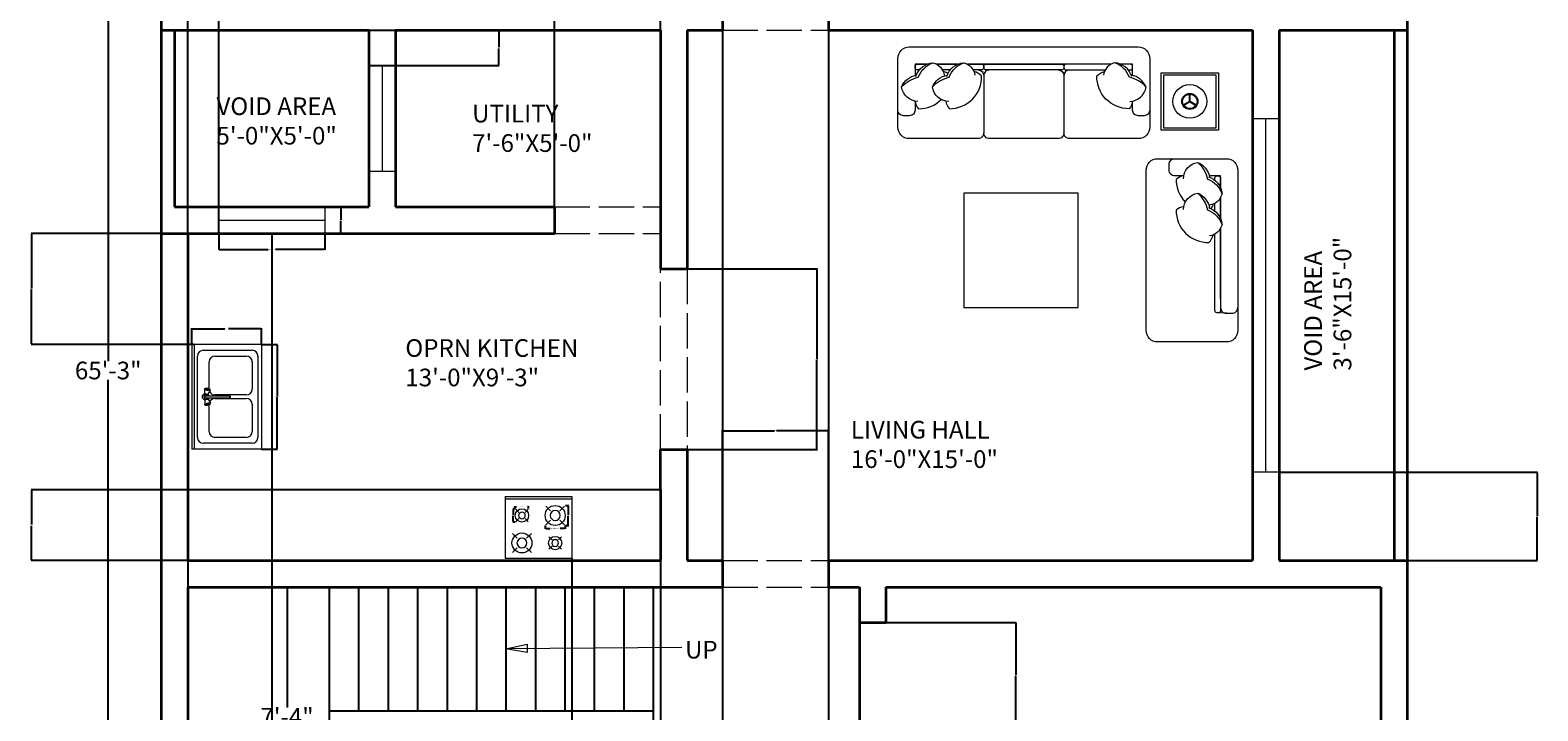
# Model space of a CAD drawing. Units: inches. Extents: x -10 to 502, y -868 to 56.
# Tile 9 of 14: x -10 to 502, y -495 to -264. Entities that reach past the tile are written whole.
import ezdxf

# ---------------------------------------------------------------- set-up
doc = ezdxf.new("R2010")
doc.units = ezdxf.units.IN
doc.header["$MEASUREMENT"] = 0
doc.linetypes.add('ACAD_ISO02W100', pattern=[15, 12, -3])
for name, color, linetype, lineweight in [('A-ANNO-DIMS', 2, 'Continuous', 18), ('A-ANNO-SYMB', 7, 'Continuous', 18), ('A-ANNO-TEXT', 7, 'Continuous', 18), ('A-AREA-IDEN', 7, 'Continuous', 18), ('A-EQPM', 8, 'Continuous', 18), ('A-FLOR-CASE', 8, 'Continuous', 18), ('A-FLOR-FIXT', 8, 'Continuous', 18), ('A-FLOR-STRS', 7, 'Continuous', 25), ('A-FURN', 8, 'Continuous', 13), ('A-GLAZ', 162, 'Continuous', 18), ('A-WALL', 7, 'Continuous', 35), ('A-WALL-OVHD', 7, 'ACAD_ISO02W100', 18)]:
    doc.layers.add(name, color=color, linetype=linetype, lineweight=lineweight)
doc.styles.get("Standard").update_dxf_attribs({"font": 'arial.ttf'})
doc.dimstyles.get("Standard").update_dxf_attribs({"dimtxt": 0.18, "dimasz": 0.18, "dimexe": 0.18, "dimexo": 0.0625, "dimgap": 0.09, "dimtad": 0, "dimtih": 1, "dimtoh": 1, "dimdec": 0, "dimzin": 0, "dimdsep": 46, "dimlunit": 3, "dimtxsty": 'Standard', "dimcen": 0.09, "dimadec": 0, "dimazin": 0, "dimtfac": 1, "dimtdec": 0, "dimtofl": 0, "dimtmove": 0, "dimatfit": 3, "dimfxl": 1, "dimtolj": 1, "dimtzin": 0, "dimarcsym": 0})

# ---------------------------------------------------------------- blocks, each defined once
blk = doc.blocks.new('*D2')
at = {"layer": 'A-ANNO-DIMS', "color": 0, "lineweight": -2, "transparency": 16777216}
for p, q in [((34.89, 12.15), (16.75, 12.15)), ((16.93, 11.97), (16.93, -376.2)), ((16.93, -770.67), (16.93, -382.51)), ((34.89, -770.85), (16.75, -770.85))]:
    blk.add_line(p, q, dxfattribs=at)
at = {"layer": 'A-ANNO-DIMS', "color": 0, "transparency": 16777216}
for points in [[(16.9, 11.97), (16.96, 11.97), (16.93, 12.15)], [(16.9, -770.67), (16.96, -770.67), (16.93, -770.85)]]:
    blk.add_solid(points, dxfattribs=at)
at = {"layer": 'Defpoints', "color": 0, "transparency": 16777216}
for p in [(34.95, 12.15), (16.93, -770.85), (34.95, -770.85)]:
    blk.add_point(p, dxfattribs=at)
at = {"layer": 'A-ANNO-DIMS', "color": 0, "transparency": 16777216, "insert": (16.93, -379.35), "char_height": 6, "attachment_point": 5}
blk.add_mtext('\\A1;65\'-3"', dxfattribs=at)
blk = doc.blocks.new('М07 600х900')
for p, q in [((0, 600), (-900, 600)), ((-900, 0), (-900, 600)), ((-900, 0), (-900, 600)), ((0, 580), (-900, 580)), ((-800, 550), (-100, 550)), ((0, 0), (0, 600)), ((0, 0), (0, 600)), ((-850, 80), (-850, 500)), ((-800, 130), (-800, 400)), ((-750, 450), (-519, 450)), ((-525, 477), (-524, 480)), ((-525, 472), (-525, 477)), ((-524, 466), (-525, 472)), ((-521, 486), (-524, 480)), ((-524, 480), (-522, 481)), ((-523, 460), (-524, 466)), ((-521, 455), (-523, 460)), ((-522, 481), (-520, 481)), ((-521, 486), (-519, 487)), ((-519, 449), (-521, 455)), ((-520, 481), (-518, 479)), ((-480, 488), (-519, 487)), ((-519, 487), (-516, 487)), ((-516, 445), (-519, 449)), ((-518, 479), (-515, 475)), ((-516, 487), (-513, 484)), ((-514, 443), (-516, 445)), ((-515, 475), (-513, 470)), ((-509, 440), (-514, 443)), ((-512, 443), (-514, 443)), ((-513, 484), (-510, 479)), ((-513, 470), (-511, 464)), ((-510, 444), (-512, 443)), ((-511, 464), (-510, 458)), ((-510, 479), (-507, 473)), ((-510, 458), (-509, 452)), ((-509, 447), (-510, 444)), ((-509, 452), (-509, 447)), ((-506, 439), (-509, 440)), ((-507, 473), (-505, 465)), ((-472, 459), (-506, 439)), ((-504, 441), (-506, 439)), ((-505, 465), (-503, 458)), ((-503, 445), (-504, 441)), ((-503, 458), (-503, 451)), ((-503, 451), (-503, 445)), ((-480, 488), (-478, 487)), ((-478, 487), (-476, 486)), ((-477, 489), (-473, 496)), ((-477, 486), (-477, 489)), ((-461, 489), (-476, 485)), ((-476, 486), (-474, 483)), ((-474, 483), (-473, 479)), ((-473, 496), (-466, 503)), ((-473, 479), (-471, 474)), ((-471, 460), (-472, 459)), ((-471, 474), (-470, 470)), ((-470, 462), (-471, 460)), ((-470, 470), (-470, 466)), ((-470, 466), (-470, 462)), ((-458, 465), (-470, 462)), ((-466, 457), (-470, 461)), ((-466, 503), (-459, 507)), ((-459, 453), (-466, 457)), ((-465, 480), (-462, 489)), ((-462, 471), (-465, 480)), ((-465, 400), (-465, 130)), ((-462, 489), (-455, 494)), ((-458, 469), (-462, 471)), ((-459, 507), (-450, 508)), ((-458, 453), (-459, 453)), ((-458, 480), (-457, 485)), ((-458, 480), (-458, 280)), ((-457, 485), (-453, 488)), ((-455, 494), (-445, 494)), ((-453, 488), (-447, 488)), ((-450, 508), (-441, 507)), ((-447, 488), (-443, 485)), ((-445, 494), (-438, 489)), ((-443, 485), (-442, 480)), ((-442, 480), (-442, 280)), ((-438, 471), (-442, 469)), ((-442, 465), (-430, 462)), ((-441, 453), (-442, 453)), ((-441, 507), (-434, 503)), ((-434, 457), (-441, 453)), ((-439, 489), (-424, 485)), ((-438, 489), (-435, 480)), ((-435, 480), (-438, 471)), ((-435, 130), (-435, 400)), ((-434, 503), (-427, 496)), ((-430, 461), (-434, 457)), ((-430, 470), (-429, 474)), ((-430, 466), (-430, 470)), ((-430, 462), (-430, 466)), ((-429, 460), (-430, 462)), ((-429, 474), (-427, 479)), ((-428, 459), (-429, 460)), ((-428, 459), (-394, 439)), ((-427, 496), (-423, 489)), ((-427, 479), (-426, 483)), ((-426, 483), (-424, 486)), ((-424, 486), (-422, 487)), ((-423, 489), (-423, 486)), ((-422, 487), (-420, 488)), ((-420, 488), (-381, 487)), ((-397, 458), (-395, 465)), ((-397, 451), (-397, 458)), ((-397, 445), (-397, 451)), ((-396, 441), (-397, 445)), ((-394, 439), (-396, 441)), ((-395, 465), (-393, 473)), ((-391, 440), (-394, 439)), ((-393, 473), (-390, 479)), ((-391, 452), (-390, 458)), ((-391, 447), (-391, 452)), ((-390, 444), (-391, 447)), ((-391, 440), (-386, 443)), ((-390, 479), (-387, 484)), ((-390, 458), (-389, 464)), ((-388, 443), (-390, 444)), ((-389, 464), (-387, 470)), ((-386, 443), (-388, 443)), ((-387, 484), (-384, 487)), ((-387, 470), (-385, 475)), ((-384, 445), (-386, 443)), ((-385, 475), (-382, 479)), ((-384, 487), (-381, 487)), ((-381, 449), (-384, 445)), ((-382, 479), (-380, 481)), ((-381, 487), (-379, 486)), ((-379, 455), (-381, 449)), ((-381, 450), (-150, 450)), ((-380, 481), (-378, 481)), ((-379, 486), (-376, 480)), ((-377, 460), (-379, 455)), ((-378, 481), (-376, 480)), ((-376, 466), (-377, 460)), ((-376, 480), (-375, 477)), ((-375, 472), (-376, 466)), ((-375, 477), (-375, 472)), ((-100, 400), (-100, 130)), ((-50, 500), (-50, 80)), ((-458, 286), (-460, 280)), ((-460, 280), (-458, 274)), ((-458, 280), (-457, 275)), ((-458, 274), (-457, 270)), ((-458, 274), (-453, 271)), ((-457, 275), (-453, 272)), ((-457, 270), (-453, 267)), ((-453, 272), (-447, 272)), ((-453, 271), (-447, 271)), ((-453, 267), (-447, 267)), ((-447, 272), (-443, 275)), ((-447, 271), (-442, 274)), ((-447, 267), (-443, 270)), ((-443, 275), (-442, 280)), ((-442, 274), (-443, 270)), ((-440, 280), (-442, 286)), ((-442, 274), (-440, 280)), ((0, 0), (-900, 0)), ((-100, 30), (-800, 30)), ((-515, 80), (-750, 80)), ((-150, 80), (-385, 80))]:
    blk.add_line(p, q)
for centre, start, end in [((-800, 500), 90, 180), ((-100, 500), 0, 90), ((-750, 400), 90, 180), ((-515, 400), 0, 65.8874), ((-385, 400), 114.1126, 180), ((-150, 400), 0, 90), ((-750, 130), 180, 270), ((-515, 130), 270, 0), ((-385, 130), 180, 270), ((-150, 130), 270, 0), ((-800, 80), 180, 270), ((-100, 80), 270, 0)]:
    blk.add_arc(centre, 50, start, end)
for p in [(-515, 80), (-150, 80), (-100, 30)]:
    blk.add_point(p)
blk = doc.blocks.new('*D6')
at = {"layer": 'A-ANNO-DIMS', "color": 0, "lineweight": -2, "transparency": 16777216}
for p, q in [((76.89, -452.85), (77.81, -452.85)), ((77.63, -453.03), (77.63, -493.76)), ((77.63, -540.67), (77.63, -499.94)), ((76.89, -540.85), (77.81, -540.85))]:
    blk.add_line(p, q, dxfattribs=at)
at = {"layer": 'A-ANNO-DIMS', "color": 0, "transparency": 16777216}
for points in [[(77.6, -453.03), (77.66, -453.03), (77.63, -452.85)], [(77.6, -540.67), (77.66, -540.67), (77.63, -540.85)]]:
    blk.add_solid(points, dxfattribs=at)
at = {"layer": 'Defpoints', "color": 0, "transparency": 16777216}
for p in [(76.83, -452.85), (76.83, -540.85), (77.63, -540.85)]:
    blk.add_point(p, dxfattribs=at)
at = {"layer": 'A-ANNO-DIMS', "color": 0, "transparency": 16777216, "insert": (77.63, -496.85), "char_height": 6, "attachment_point": 5}
blk.add_mtext('\\A1;7\'-4"', dxfattribs=at)
blk = doc.blocks.new('WIN-36IN')
for p, q in [((0, 9), (36, 9)), ((0, 0), (0, 9)), ((36, 9), (36, 0)), ((0, 4.5), (36, 4.5)), ((36, 0), (0, 0))]:
    blk.add_line(p, q)
blk = doc.blocks.new('WIN-120IN')
for p, q in [((0, 9), (120, 9)), ((0, 0), (0, 9)), ((120, 9), (120, 0)), ((0, 4.5), (120, 4.5)), ((120, 0), (0, 0))]:
    blk.add_line(p, q)
blk = doc.blocks.new('COOKTOP-BURNER-SMALL')
for p, q in [((1.19, 3.32), (0.13, 4.39)), ((1.19, 1.19), (0.13, 0.13)), ((3.32, 3.32), (4.39, 4.39)), ((3.32, 1.19), (4.39, 0.13))]:
    blk.add_line(p, q)
blk.add_circle((2.26, 2.26), 2.26)
for start, end in [(0, 180), (180, 0)]:
    blk.add_arc((2.26, 2.26), 1.13, start, end)
blk = doc.blocks.new('COOKTOP-BURNER-LARGE')
for p, q in [((1.79, 4.98), (0.19, 6.58)), ((4.98, 4.98), (6.58, 6.58)), ((1.79, 1.79), (0.19, 0.19)), ((4.98, 1.79), (6.58, 0.19))]:
    blk.add_line(p, q)
blk.add_circle((3.39, 3.39), 3.39)
for start, end in [(0, 180), (180, 0)]:
    blk.add_arc((3.39, 3.39), 1.69, start, end)
blk = doc.blocks.new('*D17')
at = {"layer": 'A-ANNO-DIMS', "color": 0, "lineweight": -2, "transparency": 16777216}
for p, q in [((54.45, -332.92), (54.45, -338.43)), ((90.45, -332.92), (90.45, -338.43)), ((54.63, -338.25), (71.22, -338.25)), ((90.27, -338.25), (73.68, -338.25))]:
    blk.add_line(p, q, dxfattribs=at)
at = {"layer": 'A-ANNO-DIMS', "color": 0, "transparency": 16777216}
for points in [[(54.63, -338.22), (54.63, -338.28), (54.45, -338.25)], [(90.27, -338.22), (90.27, -338.28), (90.45, -338.25)]]:
    blk.add_solid(points, dxfattribs=at)
at = {"layer": 'Defpoints', "color": 0, "transparency": 16777216}
for p in [(54.45, -332.85), (90.45, -332.85), (90.45, -338.25)]:
    blk.add_point(p, dxfattribs=at)
at = {"layer": 'A-ANNO-DIMS', "color": 0, "transparency": 16777216, "insert": (72.45, -338.25), "char_height": 0.18, "attachment_point": 5}
blk.add_mtext('\\A1;WINDOW 3\'-0" TYP.', dxfattribs=at)
blk = doc.blocks.new('*D18')
at = {"layer": 'A-ANNO-DIMS', "color": 0, "lineweight": -2, "transparency": 16777216}
for p, q in [((90.51, -323.85), (96.03, -323.85)), ((95.85, -324.03), (95.85, -328.17)), ((95.85, -332.67), (95.85, -328.53)), ((90.51, -332.85), (96.03, -332.85))]:
    blk.add_line(p, q, dxfattribs=at)
at = {"layer": 'A-ANNO-DIMS', "color": 0, "transparency": 16777216}
for points in [[(95.82, -324.03), (95.88, -324.03), (95.85, -323.85)], [(95.82, -332.67), (95.88, -332.67), (95.85, -332.85)]]:
    blk.add_solid(points, dxfattribs=at)
at = {"layer": 'Defpoints', "color": 0, "transparency": 16777216}
for p in [(90.45, -323.85), (95.85, -323.85), (90.45, -332.85)]:
    blk.add_point(p, dxfattribs=at)
at = {"layer": 'A-ANNO-DIMS', "color": 0, "transparency": 16777216, "insert": (95.85, -328.35), "char_height": 0.18, "attachment_point": 5}
blk.add_mtext('\\A1;0\'-9" TYP.', dxfattribs=at)
blk = doc.blocks.new('*D33')
at = {"layer": 'A-ANNO-DIMS', "color": 0, "lineweight": -2, "transparency": 16777216}
for p, q in [((69.01, -370.51), (74.45, -370.51)), ((74.27, -370.69), (74.27, -388.07)), ((74.27, -405.82), (74.27, -388.44)), ((69.01, -406), (74.45, -406))]:
    blk.add_line(p, q, dxfattribs=at)
at = {"layer": 'A-ANNO-DIMS', "color": 0, "transparency": 16777216}
for points in [[(74.24, -370.69), (74.3, -370.69), (74.27, -370.51)], [(74.24, -405.82), (74.3, -405.82), (74.27, -406)]]:
    blk.add_solid(points, dxfattribs=at)
at = {"layer": 'Defpoints', "color": 0, "transparency": 16777216}
for p in [(68.94, -370.51), (74.27, -370.51), (68.94, -406)]:
    blk.add_point(p, dxfattribs=at)
at = {"layer": 'A-ANNO-DIMS', "color": 0, "transparency": 16777216, "insert": (74.27, -388.26), "char_height": 0.18, "attachment_point": 5}
blk.add_mtext('\\A1;SINK 2\'-11 1/2"', dxfattribs=at)
blk = doc.blocks.new('*D34')
at = {"layer": 'A-ANNO-DIMS', "color": 0, "lineweight": -2, "transparency": 16777216}
for p, q in [((45.28, -370.45), (45.28, -365)), ((45.46, -365.18), (56.51, -365.18)), ((68.76, -365.18), (57.71, -365.18)), ((68.94, -370.45), (68.94, -365))]:
    blk.add_line(p, q, dxfattribs=at)
at = {"layer": 'A-ANNO-DIMS', "color": 0, "transparency": 16777216}
for points in [[(45.46, -365.15), (45.46, -365.21), (45.28, -365.18)], [(68.76, -365.15), (68.76, -365.21), (68.94, -365.18)]]:
    blk.add_solid(points, dxfattribs=at)
at = {"layer": 'Defpoints', "color": 0, "transparency": 16777216}
for p in [(45.28, -365.18), (45.28, -370.51), (68.94, -370.51)]:
    blk.add_point(p, dxfattribs=at)
at = {"layer": 'A-ANNO-DIMS', "color": 0, "transparency": 16777216, "insert": (57.11, -365.18), "char_height": 0.18, "attachment_point": 5}
blk.add_mtext('\\A1;1\'-11 1/2"', dxfattribs=at)
blk = doc.blocks.new('*D37')
at = {"layer": 'A-ANNO-DIMS', "color": 0, "lineweight": -2, "transparency": 16777216}
for p, q in [((155.13, -426.23), (155.13, -425.44)), ((155.31, -425.62), (155.53, -425.62)), ((159.46, -425.62), (159.25, -425.62)), ((159.64, -426.23), (159.64, -425.44))]:
    blk.add_line(p, q, dxfattribs=at)
at = {"layer": 'A-ANNO-DIMS', "color": 0, "transparency": 16777216}
for points in [[(155.31, -425.59), (155.31, -425.65), (155.13, -425.62)], [(159.46, -425.59), (159.46, -425.65), (159.64, -425.62)]]:
    blk.add_solid(points, dxfattribs=at)
at = {"layer": 'Defpoints', "color": 0, "transparency": 16777216}
for p in [(155.13, -426.29), (159.64, -425.62), (159.64, -426.29)]:
    blk.add_point(p, dxfattribs=at)
at = {"layer": 'A-ANNO-DIMS', "color": 0, "transparency": 16777216, "insert": (157.39, -425.62), "char_height": 0.18, "attachment_point": 5}
blk.add_mtext('\\A1;SMALL BURNER 0\'-4 1/2" TYP.', dxfattribs=at)
blk = doc.blocks.new('*D38')
at = {"layer": 'A-ANNO-DIMS', "color": 0, "lineweight": -2, "transparency": 16777216}
for p, q in [((155.07, -426.29), (154.27, -426.29)), ((154.45, -426.47), (154.45, -428.37)), ((154.45, -430.63), (154.45, -428.73)), ((155.07, -430.81), (154.27, -430.81))]:
    blk.add_line(p, q, dxfattribs=at)
at = {"layer": 'A-ANNO-DIMS', "color": 0, "transparency": 16777216}
for points in [[(154.42, -426.47), (154.48, -426.47), (154.45, -426.29)], [(154.42, -430.63), (154.48, -430.63), (154.45, -430.81)]]:
    blk.add_solid(points, dxfattribs=at)
at = {"layer": 'Defpoints', "color": 0, "transparency": 16777216}
for p in [(154.45, -426.29), (155.13, -426.29), (155.13, -430.81)]:
    blk.add_point(p, dxfattribs=at)
at = {"layer": 'A-ANNO-DIMS', "color": 0, "transparency": 16777216, "insert": (154.45, -428.55), "char_height": 0.18, "attachment_point": 5}
blk.add_mtext('\\A1;0\'-4 1/2" TYP.', dxfattribs=at)
blk = doc.blocks.new('*D39')
at = {"layer": 'A-ANNO-DIMS', "color": 0, "lineweight": -2, "transparency": 16777216}
for p, q in [((165.29, -432), (165.29, -433.13)), ((165.47, -432.95), (167.01, -432.95)), ((171.88, -432.95), (170.34, -432.95)), ((172.06, -432), (172.06, -433.13))]:
    blk.add_line(p, q, dxfattribs=at)
at = {"layer": 'A-ANNO-DIMS', "color": 0, "transparency": 16777216}
for points in [[(165.47, -432.92), (165.47, -432.98), (165.29, -432.95)], [(171.88, -432.92), (171.88, -432.98), (172.06, -432.95)]]:
    blk.add_solid(points, dxfattribs=at)
at = {"layer": 'Defpoints', "color": 0, "transparency": 16777216}
for p in [(165.29, -431.94), (165.29, -432.95), (172.06, -431.94)]:
    blk.add_point(p, dxfattribs=at)
at = {"layer": 'A-ANNO-DIMS', "color": 0, "transparency": 16777216, "insert": (168.68, -432.95), "char_height": 0.18, "attachment_point": 5}
blk.add_mtext('\\A1;LARGE BURNER 0\'-7" TYP.', dxfattribs=at)
blk = doc.blocks.new('*D40')
at = {"layer": 'A-ANNO-DIMS', "color": 0, "lineweight": -2, "transparency": 16777216}
for p, q in [((172.12, -425.16), (173.26, -425.16)), ((173.08, -425.34), (173.08, -428.37)), ((173.08, -431.76), (173.08, -428.73)), ((172.12, -431.94), (173.26, -431.94))]:
    blk.add_line(p, q, dxfattribs=at)
at = {"layer": 'A-ANNO-DIMS', "color": 0, "transparency": 16777216}
for points in [[(173.05, -425.34), (173.11, -425.34), (173.08, -425.16)], [(173.05, -431.76), (173.11, -431.76), (173.08, -431.94)]]:
    blk.add_solid(points, dxfattribs=at)
at = {"layer": 'Defpoints', "color": 0, "transparency": 16777216}
for p in [(172.06, -425.16), (172.06, -431.94), (173.08, -431.94)]:
    blk.add_point(p, dxfattribs=at)
at = {"layer": 'A-ANNO-DIMS', "color": 0, "transparency": 16777216, "insert": (173.08, -428.55), "char_height": 0.18, "attachment_point": 5}
blk.add_mtext('\\A1;0\'-7" TYP.', dxfattribs=at)
blk = doc.blocks.new('*D48')
at = {"layer": 'A-ANNO-DIMS', "color": 0, "lineweight": -2, "transparency": 16777216}
for p, q in [((43.95, -332.92), (43.95, -846.58)), ((72.45, -332.92), (72.45, -846.58)), ((44.13, -846.4), (57.66, -846.4)), ((72.27, -846.4), (58.74, -846.4))]:
    blk.add_line(p, q, dxfattribs=at)
at = {"layer": 'A-ANNO-DIMS', "color": 0, "transparency": 16777216}
for points in [[(44.13, -846.37), (44.13, -846.43), (43.95, -846.4)], [(72.27, -846.37), (72.27, -846.43), (72.45, -846.4)]]:
    blk.add_solid(points, dxfattribs=at)
at = {"layer": 'Defpoints', "color": 0, "transparency": 16777216}
for p in [(43.95, -332.85), (72.45, -332.85), (72.45, -846.4)]:
    blk.add_point(p, dxfattribs=at)
at = {"layer": 'A-ANNO-DIMS', "color": 0, "transparency": 16777216, "insert": (58.2, -846.4), "char_height": 0.18, "attachment_point": 5}
blk.add_mtext('\\A1;2\'-4 1/2"', dxfattribs=at)
blk = doc.blocks.new('*D49')
at = {"layer": 'A-ANNO-DIMS', "color": 0, "lineweight": -2, "transparency": 16777216}
for p, q in [((204.39, -419.85), (-9.28, -419.85)), ((-9.1, -420.03), (-9.1, -431.67)), ((-9.1, -443.67), (-9.1, -432.03)), ((204.39, -443.85), (-9.28, -443.85))]:
    blk.add_line(p, q, dxfattribs=at)
at = {"layer": 'A-ANNO-DIMS', "color": 0, "transparency": 16777216}
for points in [[(-9.13, -420.03), (-9.07, -420.03), (-9.1, -419.85)], [(-9.13, -443.67), (-9.07, -443.67), (-9.1, -443.85)]]:
    blk.add_solid(points, dxfattribs=at)
at = {"layer": 'Defpoints', "color": 0, "transparency": 16777216}
for p in [(204.45, -419.85), (-9.1, -443.85), (204.45, -443.85)]:
    blk.add_point(p, dxfattribs=at)
at = {"layer": 'A-ANNO-DIMS', "color": 0, "transparency": 16777216, "insert": (-9.1, -431.85), "char_height": 0.18, "attachment_point": 5}
blk.add_mtext('\\A1;2\'-0"', dxfattribs=at)
blk = doc.blocks.new('*D52')
at = {"layer": 'A-ANNO-DIMS', "color": 0, "lineweight": -2, "transparency": 16777216}
for p, q in [((414.51, -413.85), (502.18, -413.85)), ((502, -414.03), (502, -428.67)), ((502, -443.67), (502, -429.03)), ((414.51, -443.85), (502.18, -443.85))]:
    blk.add_line(p, q, dxfattribs=at)
at = {"layer": 'A-ANNO-DIMS', "color": 0, "transparency": 16777216}
for points in [[(501.97, -414.03), (502.03, -414.03), (502, -413.85)], [(501.97, -443.67), (502.03, -443.67), (502, -443.85)]]:
    blk.add_solid(points, dxfattribs=at)
at = {"layer": 'Defpoints', "color": 0, "transparency": 16777216}
for p in [(414.45, -413.85), (414.45, -443.85), (502, -443.85)]:
    blk.add_point(p, dxfattribs=at)
at = {"layer": 'A-ANNO-DIMS', "color": 0, "transparency": 16777216, "insert": (502, -428.85), "char_height": 0.18, "attachment_point": 5}
blk.add_mtext('\\A1;2\'-6"', dxfattribs=at)
blk = doc.blocks.new('*D53')
at = {"layer": 'A-ANNO-DIMS', "color": 0, "lineweight": -2, "transparency": 16777216}
for p, q in [((174.32, -443.06), (174.32, -846.58)), ((204.45, -443.92), (204.45, -846.58)), ((174.5, -846.4), (189.05, -846.4)), ((204.27, -846.4), (189.72, -846.4))]:
    blk.add_line(p, q, dxfattribs=at)
at = {"layer": 'A-ANNO-DIMS', "color": 0, "transparency": 16777216}
for points in [[(174.5, -846.37), (174.5, -846.43), (174.32, -846.4)], [(204.27, -846.37), (204.27, -846.43), (204.45, -846.4)]]:
    blk.add_solid(points, dxfattribs=at)
at = {"layer": 'Defpoints', "color": 0, "transparency": 16777216}
for p in [(174.32, -443), (204.45, -443.85), (204.45, -846.4)]:
    blk.add_point(p, dxfattribs=at)
at = {"layer": 'A-ANNO-DIMS', "color": 0, "transparency": 16777216, "insert": (189.39, -846.4), "char_height": 0.18, "attachment_point": 5}
blk.add_mtext('\\A1;2\'-6"', dxfattribs=at)
blk = doc.blocks.new('*D54')
at = {"layer": 'A-ANNO-DIMS', "color": 0, "lineweight": -2, "transparency": 16777216}
for p, q in [((213.51, -344.85), (257.68, -344.85)), ((257.5, -345.03), (257.5, -375.35)), ((257.5, -406.03), (257.5, -375.72)), ((213.51, -406.21), (257.68, -406.21))]:
    blk.add_line(p, q, dxfattribs=at)
at = {"layer": 'A-ANNO-DIMS', "color": 0, "transparency": 16777216}
for points in [[(257.47, -345.03), (257.53, -345.03), (257.5, -344.85)], [(257.47, -406.03), (257.53, -406.03), (257.5, -406.21)]]:
    blk.add_solid(points, dxfattribs=at)
at = {"layer": 'Defpoints', "color": 0, "transparency": 16777216}
for p in [(213.45, -344.85), (213.45, -406.21), (257.5, -406.21)]:
    blk.add_point(p, dxfattribs=at)
at = {"layer": 'A-ANNO-DIMS', "color": 0, "transparency": 16777216, "insert": (257.5, -375.53), "char_height": 0.18, "attachment_point": 5}
blk.add_mtext('\\A1;5\'-1 1/2"', dxfattribs=at)
blk = doc.blocks.new('*D55')
at = {"layer": 'A-ANNO-DIMS', "color": 0, "lineweight": -2, "transparency": 16777216}
for p, q in [((225.45, -443.79), (225.45, -399.62)), ((225.63, -399.8), (243.12, -399.8)), ((261.27, -399.8), (243.78, -399.8)), ((261.45, -443.79), (261.45, -399.62))]:
    blk.add_line(p, q, dxfattribs=at)
at = {"layer": 'A-ANNO-DIMS', "color": 0, "transparency": 16777216}
for points in [[(225.63, -399.77), (225.63, -399.83), (225.45, -399.8)], [(261.27, -399.77), (261.27, -399.83), (261.45, -399.8)]]:
    blk.add_solid(points, dxfattribs=at)
at = {"layer": 'Defpoints', "color": 0, "transparency": 16777216}
for p in [(261.45, -399.8), (225.45, -443.85), (261.45, -443.85)]:
    blk.add_point(p, dxfattribs=at)
at = {"layer": 'A-ANNO-DIMS', "color": 0, "transparency": 16777216, "insert": (243.45, -399.8), "char_height": 0.18, "attachment_point": 5}
blk.add_mtext('\\A1;3\'-0"', dxfattribs=at)
blk = doc.blocks.new('*D58')
at = {"layer": 'A-ANNO-DIMS', "color": 0, "lineweight": -2, "transparency": 16777216}
for p, q in [((281.01, -464.85), (325.18, -464.85)), ((325, -465.03), (325, -482.67)), ((325, -500.67), (325, -483.03)), ((281.01, -500.85), (325.18, -500.85))]:
    blk.add_line(p, q, dxfattribs=at)
at = {"layer": 'A-ANNO-DIMS', "color": 0, "transparency": 16777216}
for points in [[(324.97, -465.03), (325.03, -465.03), (325, -464.85)], [(324.97, -500.67), (325.03, -500.67), (325, -500.85)]]:
    blk.add_solid(points, dxfattribs=at)
at = {"layer": 'Defpoints', "color": 0, "transparency": 16777216}
for p in [(280.95, -464.85), (280.95, -500.85), (325, -500.85)]:
    blk.add_point(p, dxfattribs=at)
at = {"layer": 'A-ANNO-DIMS', "color": 0, "transparency": 16777216, "insert": (325, -482.85), "char_height": 0.18, "attachment_point": 5}
blk.add_mtext('\\A1;3\'-0"', dxfattribs=at)
blk = doc.blocks.new('*D59')
at = {"layer": 'A-ANNO-DIMS', "color": 0, "lineweight": -2, "transparency": 16777216}
for p, q in [((43.89, -332.85), (-9.28, -332.85)), ((-9.1, -333.03), (-9.1, -351.5)), ((-9.1, -370.33), (-9.1, -351.86)), ((46.01, -370.51), (-9.28, -370.51))]:
    blk.add_line(p, q, dxfattribs=at)
at = {"layer": 'A-ANNO-DIMS', "color": 0, "transparency": 16777216}
for points in [[(-9.13, -333.03), (-9.07, -333.03), (-9.1, -332.85)], [(-9.13, -370.33), (-9.07, -370.33), (-9.1, -370.51)]]:
    blk.add_solid(points, dxfattribs=at)
at = {"layer": 'Defpoints', "color": 0, "transparency": 16777216}
for p in [(43.95, -332.85), (-9.1, -370.51), (46.07, -370.51)]:
    blk.add_point(p, dxfattribs=at)
at = {"layer": 'A-ANNO-DIMS', "color": 0, "transparency": 16777216, "insert": (-9.1, -351.68), "char_height": 0.18, "attachment_point": 5}
blk.add_mtext('\\A1;3\'-1 1/2"', dxfattribs=at)
blk = doc.blocks.new('*D60')
at = {"layer": 'A-ANNO-DIMS', "color": 0, "lineweight": -2, "transparency": 16777216}
for p, q in [((168.45, -332.79), (168.45, 56.38)), ((204.45, -332.79), (204.45, 56.38)), ((168.63, 56.2), (186.12, 56.2)), ((204.27, 56.2), (186.78, 56.2))]:
    blk.add_line(p, q, dxfattribs=at)
at = {"layer": 'A-ANNO-DIMS', "color": 0, "transparency": 16777216}
for points in [[(168.63, 56.23), (168.63, 56.17), (168.45, 56.2)], [(204.27, 56.23), (204.27, 56.17), (204.45, 56.2)]]:
    blk.add_solid(points, dxfattribs=at)
at = {"layer": 'Defpoints', "color": 0, "transparency": 16777216}
for p in [(204.45, 56.2), (168.45, -332.85), (204.45, -332.85)]:
    blk.add_point(p, dxfattribs=at)
at = {"layer": 'A-ANNO-DIMS', "color": 0, "transparency": 16777216, "insert": (186.45, 56.2), "char_height": 0.18, "attachment_point": 5}
blk.add_mtext('\\A1;3\'-0"', dxfattribs=at)
blk = doc.blocks.new('*D62')
at = {"layer": 'A-ANNO-DIMS', "color": 0, "lineweight": -2, "transparency": 16777216}
for p, q in [((105.51, -263.85), (149.68, -263.85)), ((149.5, -264.03), (149.5, -269.67)), ((149.5, -275.67), (149.5, -270.03)), ((105.51, -275.85), (149.68, -275.85))]:
    blk.add_line(p, q, dxfattribs=at)
at = {"layer": 'A-ANNO-DIMS', "color": 0, "transparency": 16777216}
for points in [[(149.47, -264.03), (149.53, -264.03), (149.5, -263.85)], [(149.47, -275.67), (149.53, -275.67), (149.5, -275.85)]]:
    blk.add_solid(points, dxfattribs=at)
at = {"layer": 'Defpoints', "color": 0, "transparency": 16777216}
for p in [(105.45, -263.85), (105.45, -275.85), (149.5, -275.85)]:
    blk.add_point(p, dxfattribs=at)
at = {"layer": 'A-ANNO-DIMS', "color": 0, "transparency": 16777216, "insert": (149.5, -269.85), "char_height": 0.18, "attachment_point": 5}
blk.add_mtext('\\A1;1\'-0"', dxfattribs=at)
blk = doc.blocks.new('*D64')
at = {"layer": 'A-ANNO-DIMS', "color": 0, "lineweight": -2, "transparency": 16777216}
for p, q in [((43.95, -332.79), (43.95, 56.38)), ((54.45, -332.79), (54.45, 56.38)), ((44.13, 56.2), (48.59, 56.2)), ((54.27, 56.2), (49.81, 56.2))]:
    blk.add_line(p, q, dxfattribs=at)
at = {"layer": 'A-ANNO-DIMS', "color": 0, "transparency": 16777216}
for points in [[(44.13, 56.23), (44.13, 56.17), (43.95, 56.2)], [(54.27, 56.23), (54.27, 56.17), (54.45, 56.2)]]:
    blk.add_solid(points, dxfattribs=at)
at = {"layer": 'Defpoints', "color": 0, "transparency": 16777216}
for p in [(54.45, 56.2), (43.95, -332.85), (54.45, -332.85)]:
    blk.add_point(p, dxfattribs=at)
at = {"layer": 'A-ANNO-DIMS', "color": 0, "transparency": 16777216, "insert": (49.2, 56.2), "char_height": 0.18, "attachment_point": 5}
blk.add_mtext('\\A1;0\'-10 1/2"', dxfattribs=at)
blk = doc.blocks.new('*D65')
at = {"layer": 'A-ANNO-DIMS', "color": 0, "lineweight": -2, "transparency": 16777216}
for p, q in [((225.45, -263.92), (225.45, -846.58)), ((261.45, -263.92), (261.45, -846.58)), ((225.63, -846.4), (243.12, -846.4)), ((261.27, -846.4), (243.78, -846.4))]:
    blk.add_line(p, q, dxfattribs=at)
at = {"layer": 'A-ANNO-DIMS', "color": 0, "transparency": 16777216}
for points in [[(225.63, -846.37), (225.63, -846.43), (225.45, -846.4)], [(261.27, -846.37), (261.27, -846.43), (261.45, -846.4)]]:
    blk.add_solid(points, dxfattribs=at)
at = {"layer": 'Defpoints', "color": 0, "transparency": 16777216}
for p in [(225.45, -263.85), (261.45, -263.85), (261.45, -846.4)]:
    blk.add_point(p, dxfattribs=at)
at = {"layer": 'A-ANNO-DIMS', "color": 0, "transparency": 16777216, "insert": (243.45, -846.4), "char_height": 0.18, "attachment_point": 5}
blk.add_mtext('\\A1;3\'-0"', dxfattribs=at)

msp = doc.modelspace()

# ---------------------------------------------------------------- linework, layer by layer
at = {"layer": 'A-ANNO-SYMB'}
for p, q in [((151.95, -473.85), (159.19, -472.19)), ((211.65, -473.31), (151.95, -473.85)), ((159.19, -475.02), (151.95, -473.85)), ((159.19, -472.19), (159.19, -475.02))]:
    msp.add_line(p, q, dxfattribs=at)
at = {"layer": 'A-EQPM'}
for p, q in [((151.74, -422.15), (174.32, -422.15)), ((151.74, -422.15), (151.74, -443)), ((151.74, -422.91), (174.32, -422.91)), ((174.32, -422.15), (174.32, -443)), ((151.74, -443), (174.32, -443))]:
    msp.add_line(p, q, dxfattribs=at)
at = {"layer": 'A-FLOR-CASE'}
for p, q in [((72.45, -332.85), (72.45, -419.85)), ((72.45, -419.85), (204.45, -419.85))]:
    msp.add_line(p, q, dxfattribs=at)
at = {"layer": 'A-FLOR-STRS'}
for p, q in [((91.95, -452.85), (91.95, -498.85)), ((101.95, -452.85), (101.95, -494.85)), ((111.95, -452.85), (111.95, -494.85)), ((121.95, -452.85), (121.95, -494.85)), ((131.95, -452.85), (131.95, -494.85)), ((141.95, -452.85), (141.95, -494.85)), ((151.95, -452.85), (151.95, -494.85)), ((161.95, -452.85), (161.95, -494.85)), ((171.95, -452.85), (171.95, -494.85)), ((181.95, -452.85), (181.95, -494.85)), ((191.95, -452.85), (191.95, -494.85)), ((201.95, -452.85), (201.95, -498.85)), ((91.95, -494.85), (201.95, -494.85))]:
    msp.add_line(p, q, dxfattribs=at)
at = {"layer": 'A-FURN'}
for p, q in [((384.01, -288.03), (384.01, -285.29)), ((384.25, -288.03), (384.25, -285.29)), ((384.07, -287.92), (381.7, -289.3)), ((384.19, -288.14), (381.82, -289.51)), ((384.07, -288.14), (386.44, -289.51)), ((384.19, -287.92), (386.57, -289.3)), ((396.52, -359.95), (393.6, -359.76))]:
    msp.add_line(p, q, dxfattribs=at)
at = {"layer": 'A-FURN', "ltscale": 0.03}
for points in [[(370.52, -296.78, -0.414214), (366.64, -300.67), (343.31, -300.67, -0.414214), (341.37, -298.72, -0.414214), (339.42, -300.67), (316.1, -300.67, -0.414214), (314.15, -298.72, -0.414214), (312.21, -300.67), (288.88, -300.67, -0.414214), (285, -296.78), (285, -273.45, -0.414214), (288.88, -269.56), (366.64, -269.56, -0.414214), (370.52, -273.45)], [(373.19, -369.67, -0.414214), (369.3, -365.78), (369.3, -365.78, 0.317837), (369.3, -365.78, -0.414214), (369.3, -365.78), (369.3, -365.78, 1.186185), (369.3, -365.78, -0.414214), (369.3, -365.78), (369.3, -311.36, -0.414214), (373.19, -307.47), (396.52, -307.47, -0.414214), (400.4, -311.36), (400.4, -365.78, -0.414214), (396.52, -369.67)]]:
    msp.add_lwpolyline(points, format="xyb", close=True, dxfattribs=at)
at = {"layer": 'A-FURN'}
for points in [[(286.23, -283.15, -0.14773), (291.92, -279.81, -0.213343), (296.93, -274.91)], [(294.92, -275.4), (290.83, -275.4), (290.83, -279.22, -0.414352)], [(292.31, -277.34), (291.61, -277.34, -0.414214), (290.83, -276.56), (290.83, -276.17, -0.414214), (291.61, -275.4)], [(291.13, -279.55, -0.306663), (296.93, -274.91, -0.30633), (300.72, -279.14)], [(291.61, -275.4), (294.92, -275.4, -0.414469)], [(296.71, -283.15, -0.14773), (302.39, -279.81, -0.213343), (307.4, -274.91)], [(298.15, -275.4), (305.39, -275.4, -0.414747)], [(301.6, -279.55, -0.306663), (307.4, -274.91, -0.30633), (311.19, -279.14)], [(308.62, -275.4), (313.38, -275.4, -0.414214), (314.15, -276.17), (314.15, -276.56, -0.414214), (313.38, -277.34), (310.58, -277.34, -0.126313)], [(357.37, -275.4), (342.14, -275.4, 0.414214), (341.37, -276.17), (341.37, -276.56, 0.414214), (342.14, -277.34), (355.41, -277.34, 0.412652)], [(364.39, -279.55, 0.306663), (358.59, -274.91, 0.30633), (354.81, -279.14)], [(369.29, -283.15, 0.14773), (363.61, -279.81, 0.213343), (358.59, -274.91)], [(363.92, -275.4), (360.6, -275.4, 0.412535)], [(363.21, -277.34), (363.92, -277.34, 0.414214), (364.69, -276.56), (364.69, -276.17, 0.414214), (363.92, -275.4)], [(291.8, -288.05, -0.356772), (286.23, -283.15, -0.249542), (291.28, -279.12)], [(302.28, -288.05, -0.356772), (296.71, -283.15, -0.249542), (301.75, -279.12)], [(302.78, -277.34), (300.11, -277.34, -0.414599)], [(301.98, -278.59, 0.071865), (300.35, -277.83)], [(301.3, -287.93, 0.165541), (302.5, -290.5, 0.425989), (313.41, -279.37, 0.121523), (310.82, -277.83)], [(312.21, -277.34, -0.414214), (314.15, -279.28), (314.15, -298.72, -0.41732)], [(316.1, -277.34, 0.414214), (314.15, -279.28)], [(339.42, -277.34, -0.414214), (341.37, -279.28)], [(343.31, -277.34, 0.414214), (341.37, -279.28), (341.37, -298.72, 0.415249)], [(364.7, -287.93, -0.165541), (363.49, -290.5, -0.425989), (352.58, -279.37, -0.121523), (355.17, -277.83)], [(363.72, -288.05, 0.356772), (369.29, -283.15, 0.249542), (364.24, -279.12)], [(290.83, -287.93), (290.83, -290.95, -0.414214), (288.88, -292.89), (286.94, -292.89, -0.414214), (285, -290.95)], [(290.82, -287.93, 0.165541), (292.03, -290.5, 0.200231), (299.74, -287.37)], [(370.52, -290.95, -0.414214), (368.58, -292.89), (366.64, -292.89, -0.414214), (364.69, -290.95), (364.69, -287.93)], [(382.03, -313.3), (379.02, -313.3, -0.414214), (377.08, -311.36), (377.08, -309.41, -0.414214), (379.02, -307.47)], [(381.92, -314.28, -0.356772), (386.82, -308.71, -0.249542), (390.85, -313.75, 9.61688)], [(386.82, -308.71, -0.14773), (390.16, -314.39, -0.213343), (395.06, -319.4, -0.178662)], [(382.03, -313.3, 0.165541), (379.47, -314.5, 0.200231), (382.59, -322.21, 0.121523)], [(390.42, -313.6, -0.306663), (395.06, -319.4, -0.30633), (390.82, -323.19, 0.872847)], [(394.57, -317.39), (394.57, -313.3), (390.75, -313.3, -0.414214)], [(392.63, -314.78), (392.63, -314.08, -0.414214), (393.41, -313.3), (393.8, -313.3, -0.414214), (394.57, -314.08)], [(394.57, -314.08), (394.57, -317.39, -0.414214)], [(381.92, -324.75, -0.356772), (386.82, -319.18, -0.249542), (390.85, -324.22, 9.61688)], [(386.82, -319.18, -0.14773), (390.16, -324.86, -0.213343), (395.06, -329.87, -0.178662)], [(394.57, -320.62), (394.57, -327.86, -0.414214)], [(382.03, -323.77, 0.165541), (379.47, -324.97, 0.425989), (390.6, -335.89, 0.121523), (392.14, -333.29, -7.115464)], [(390.42, -324.07, -0.306663), (395.06, -329.87, -0.30633), (390.82, -333.66, 0.872847)], [(391.38, -324.45, 0.071865), (392.14, -322.82, -7.115464)], [(392.63, -325.25), (392.63, -322.58, -0.414214)], [(394.57, -331.09), (394.57, -358.98, -0.414214), (393.8, -359.76), (393.41, -359.76, -0.414214), (392.63, -358.98), (392.63, -333.05, -0.414214)], [(394.57, -355), (394.57, -358.01, 0.414214), (396.52, -359.95), (398.46, -359.95, 0.414214), (400.4, -358.01)]]:
    msp.add_lwpolyline(points, format="xyb", dxfattribs=at)
for points in [[(305.39, -275.4), (298.15, -275.4)], [(357.37, -275.4), (308.62, -275.4)], [(364.69, -279.22), (364.69, -275.4), (360.6, -275.4)], [(394.57, -327.86), (394.57, -320.62)], [(394.57, -355), (394.57, -331.09)]]:
    msp.add_lwpolyline(points, dxfattribs=at)
msp.add_lwpolyline([(314.93, -275.4), (340.59, -275.4, -0.414214), (341.37, -276.17), (341.37, -276.56, -0.414214), (340.59, -277.34), (314.93, -277.34, -0.414214), (314.15, -276.56), (314.15, -276.17, -0.414214)], format="xyb", close=True, dxfattribs=at)
at = {"layer": 'A-FURN', "ltscale": 0.03}
for points in [[(393.85, -297.75), (374.41, -297.75), (374.41, -278.31), (393.85, -278.31)], [(307.35, -358.01), (346.23, -358.01), (346.23, -319.13), (307.35, -319.13)]]:
    msp.add_lwpolyline(points, close=True, dxfattribs=at)
at = {"layer": 'A-FURN'}
msp.add_lwpolyline([(375.19, -296.97), (393.07, -296.97), (393.07, -279.09), (375.19, -279.09)], close=True, dxfattribs=at)
for radius in [5.73, 2.74, 2.46]:
    msp.add_circle((384.13, -288.03), radius, dxfattribs=at)
at = {"layer": 'A-WALL'}
for p, q in [((34.95, 12.15), (34.95, -770.85)), ((457.95, 3.15), (457.95, -770.85)), ((225.45, -254.85), (225.45, -263.85)), ((261.45, -254.85), (261.45, -263.85)), ((34.95, -263.85), (105.45, -263.85)), ((39.45, -263.85), (39.45, -323.85)), ((105.45, -263.85), (105.45, -323.85)), ((114.45, -263.85), (114.45, -323.85)), ((114.45, -263.85), (204.45, -263.85)), ((204.45, -263.85), (204.45, -344.85)), ((213.45, -263.85), (213.45, -344.85)), ((213.45, -263.85), (225.45, -263.85)), ((261.45, -263.85), (405.45, -263.85)), ((405.45, -263.85), (405.45, -443.85)), ((414.45, -263.85), (414.45, -443.85)), ((414.45, -263.85), (457.95, -263.85)), ((453.45, -263.85), (453.45, -443.85)), ((39.45, -323.85), (105.45, -323.85)), ((114.45, -323.85), (168.45, -323.85)), ((168.45, -323.85), (168.45, -332.85)), ((34.95, -332.85), (168.45, -332.85)), ((43.95, -332.85), (43.95, -443.85)), ((204.45, -344.85), (213.45, -344.85)), ((204.45, -419.85), (204.45, -406.21)), ((204.45, -406.21), (213.45, -406.21)), ((213.45, -406.21), (213.45, -419.85)), ((204.45, -419.85), (204.45, -443.85)), ((213.45, -419.85), (213.45, -443.85)), ((43.95, -443.85), (204.45, -443.85)), ((213.45, -443.85), (225.45, -443.85)), ((225.45, -443.85), (225.45, -452.85)), ((261.45, -443.85), (261.45, -452.85)), ((261.45, -443.85), (405.45, -443.85)), ((414.45, -443.85), (457.95, -443.85)), ((43.95, -452.85), (225.45, -452.85)), ((43.95, -452.85), (43.95, -540.85)), ((261.45, -452.85), (271.95, -452.85)), ((271.95, -452.85), (271.95, -540.85)), ((280.95, -452.85), (280.95, -464.85)), ((280.95, -452.85), (448.95, -452.85)), ((448.95, -452.85), (448.95, -644.85)), ((271.95, -464.85), (280.95, -464.85))]:
    msp.add_line(p, q, dxfattribs=at)
at = {"layer": 'A-WALL-OVHD'}
for p, q in [((225.45, -263.85), (261.45, -263.85)), ((168.45, -323.85), (204.45, -323.85)), ((168.45, -332.85), (204.45, -332.85)), ((204.45, -406.21), (204.45, -344.85)), ((213.45, -344.85), (213.45, -406.21)), ((225.45, -443.85), (261.45, -443.85)), ((225.45, -452.85), (261.45, -452.85))]:
    msp.add_line(p, q, dxfattribs=at)

# ---------------------------------------------------------------- block references
at = {"layer": 'A-EQPM'}
for name, p in [('COOKTOP-BURNER-SMALL', (155.13, -430.81)), ('COOKTOP-BURNER-LARGE', (154, -441.28))]:
    msp.add_blockref(name, p, dxfattribs=at)
at = {"layer": 'A-EQPM', "rotation": 180}
for name, p in [('COOKTOP-BURNER-LARGE', (172.06, -425.16)), ('COOKTOP-BURNER-SMALL', (170.93, -435.64))]:
    msp.add_blockref(name, p, dxfattribs=at)
at = {"layer": 'A-FLOR-FIXT', "xscale": 0.0394395368169949, "yscale": 0.0394395368169949, "zscale": 0.0394395368169949, "rotation": 90}
msp.add_blockref('М07 600х900', (68.94, -370.51), dxfattribs=at)
at = {"layer": 'A-GLAZ'}
for name, p, rotation in [('WIN-36IN', (105.45, -275.85), 270.0000000000001), ('WIN-120IN', (414.45, -413.85), 89.99999999999996)]:
    msp.add_blockref(name, p, dxfattribs=dict(at, rotation=rotation))
msp.add_blockref('WIN-36IN', (54.45, -332.85), dxfattribs=at)

# ---------------------------------------------------------------- texts
at = {"layer": 'A-ANNO-TEXT', "insert": (212.74, -471.1), "char_height": 6, "attachment_point": 1}
msp.add_mtext('UP', dxfattribs=at)
at = {"layer": 'A-AREA-IDEN', "char_height": 6, "attachment_point": 1}
for s, insert in [('VOID AREA\\P5\'-0"X5\'-0"', (53.68, -286.67)), ('UTILITY\\P7\'-6"X5\'-0"', (140.46, -289.17)), ('OPRN KITCHEN\\P13\'-0"X9\'-3"', (117.8, -368.72)), ('LIVING HALL\\P16\'-0"X15\'-0"', (269.04, -396.44))]:
    msp.add_mtext(s, dxfattribs=dict(at, insert=insert))
at = {"layer": 'A-AREA-IDEN', "insert": (422.95, -379.38), "char_height": 6, "attachment_point": 1, "rotation": 90}
msp.add_mtext_dynamic_manual_height_columns('VOID AREA\\P3\'-6"X15\'-0"', width=55.8549, gutter_width=1, heights=[21.49], dxfattribs=at)

# ---------------------------------------------------------------- dimensions: what is measured, and where the dimension line sits
at = {"layer": 'A-ANNO-DIMS'}
for base, p1, p2, picture, middle in [((54.45, 56.2), (43.95, -332.85), (54.45, -332.85), '*D64', (49.2, 56.2)), ((204.45, 56.2), (168.45, -332.85), (204.45, -332.85), '*D60', (186.45, 56.2)), ((261.45, -846.4), (225.45, -263.85), (261.45, -263.85), '*D65', (243.45, -846.4)), ((72.45, -846.4), (43.95, -332.85), (72.45, -332.85), '*D48', (58.2, -846.4)), ((261.45, -399.8), (225.45, -443.85), (261.45, -443.85), '*D55', (243.45, -399.8)), ((204.45, -846.4), (174.32, -443), (204.45, -443.85), '*D53', (189.39, -846.4))]:
    dim = msp.add_linear_dim(base=base, p1=p1, p2=p2, dimstyle='Standard', override={"dimdec": 1, "dimlfac": 1, "dimrnd": 0, "dimzin": 1, "dimdsep": 46, "dimlunit": 4, "dimfrac": 2}, dxfattribs=at)
    dim.commit()
    dim.dimension.update_dxf_attribs({"geometry": picture, "text_midpoint": middle})
for base, p1, p2, angle, override, picture, middle in [((16.93, -770.85), (34.95, 12.15), (34.95, -770.85), 90, {"dimtxt": 6, "dimclrd": 0, "dimclre": 0, "dimclrt": 0}, '*D2', (16.93, -379.35)), ((149.5, -275.85), (105.45, -263.85), (105.45, -275.85), 270, {"dimdec": 1, "dimlfac": 1, "dimrnd": 0, "dimzin": 1, "dimdsep": 46, "dimlunit": 4, "dimfrac": 2}, '*D62', (149.5, -269.85)), ((-9.1, -370.51), (43.95, -332.85), (46.07, -370.51), 90, {"dimdec": 1, "dimlfac": 1, "dimrnd": 0, "dimzin": 1, "dimdsep": 46, "dimlunit": 4, "dimfrac": 2}, '*D59', (-9.1, -351.68)), ((257.5, -406.21), (213.45, -344.85), (213.45, -406.21), 270, {"dimdec": 1, "dimlfac": 1, "dimrnd": 0, "dimzin": 1, "dimdsep": 46, "dimlunit": 4, "dimfrac": 2}, '*D54', (257.5, -375.53)), ((45.28, -365.18), (68.94, -370.51), (45.28, -370.51), 180, {"dimdec": 1, "dimlfac": 1, "dimrnd": 0, "dimzin": 1, "dimdsep": 46, "dimlunit": 4, "dimfrac": 2}, '*D34', (57.11, -365.18)), ((502, -443.85), (414.45, -413.85), (414.45, -443.85), 90, {"dimdec": 1, "dimlfac": 1, "dimrnd": 0, "dimzin": 1, "dimdsep": 46, "dimlunit": 4, "dimfrac": 2}, '*D52', (502, -428.85)), ((-9.1, -443.85), (204.45, -419.85), (204.45, -443.85), 90, {"dimdec": 1, "dimlfac": 1, "dimrnd": 0, "dimzin": 1, "dimdsep": 46, "dimlunit": 4, "dimfrac": 2}, '*D49', (-9.1, -431.85)), ((77.63, -540.85), (76.83, -452.85), (76.83, -540.85), 90, {"dimtxt": 6, "dimclrd": 0, "dimclre": 0, "dimclrt": 0}, '*D6', (77.63, -496.85)), ((325, -500.85), (280.95, -464.85), (280.95, -500.85), 270, {"dimdec": 1, "dimlfac": 1, "dimrnd": 0, "dimzin": 1, "dimdsep": 46, "dimlunit": 4, "dimfrac": 2}, '*D58', (325, -482.85))]:
    dim = msp.add_linear_dim(base=base, p1=p1, p2=p2, angle=angle, dimstyle='Standard', override=override, dxfattribs=at)
    dim.commit()
    dim.dimension.update_dxf_attribs({"geometry": picture, "text_midpoint": middle})
for base, p1, p2, angle, text, picture, middle in [((95.85, -323.85), (90.45, -332.85), (90.45, -323.85), 90, '<> TYP.', '*D18', (95.85, -328.35)), ((74.27, -370.51), (68.94, -406), (68.94, -370.51), 90, 'SINK <>', '*D33', (74.27, -388.26)), ((154.45, -426.29), (155.13, -430.81), (155.13, -426.29), 90, '<> TYP.', '*D38', (154.45, -428.55)), ((173.08, -431.94), (172.06, -425.16), (172.06, -431.94), 270, '<> TYP.', '*D40', (173.08, -428.55)), ((165.29, -432.95), (172.06, -431.94), (165.29, -431.94), 180, 'LARGE BURNER <> TYP.', '*D39', (168.68, -432.95))]:
    dim = msp.add_linear_dim(base=base, p1=p1, p2=p2, angle=angle, text=text, dimstyle='Standard', override={"dimdec": 1, "dimlfac": 1, "dimrnd": 0, "dimzin": 1, "dimdsep": 46, "dimlunit": 4, "dimfrac": 2}, dxfattribs=at)
    dim.commit()
    dim.dimension.update_dxf_attribs({"geometry": picture, "text_midpoint": middle})
for base, p1, p2, text, picture, middle in [((90.45, -338.25), (54.45, -332.85), (90.45, -332.85), 'WINDOW <> TYP.', '*D17', (72.45, -338.25)), ((159.64, -425.62), (155.13, -426.29), (159.64, -426.29), 'SMALL BURNER <> TYP.', '*D37', (157.39, -425.62))]:
    dim = msp.add_linear_dim(base=base, p1=p1, p2=p2, text=text, dimstyle='Standard', override={"dimdec": 1, "dimlfac": 1, "dimrnd": 0, "dimzin": 1, "dimdsep": 46, "dimlunit": 4, "dimfrac": 2}, dxfattribs=at)
    dim.commit()
    dim.dimension.update_dxf_attribs({"geometry": picture, "text_midpoint": middle})

doc.saveas('drawing.dxf')
